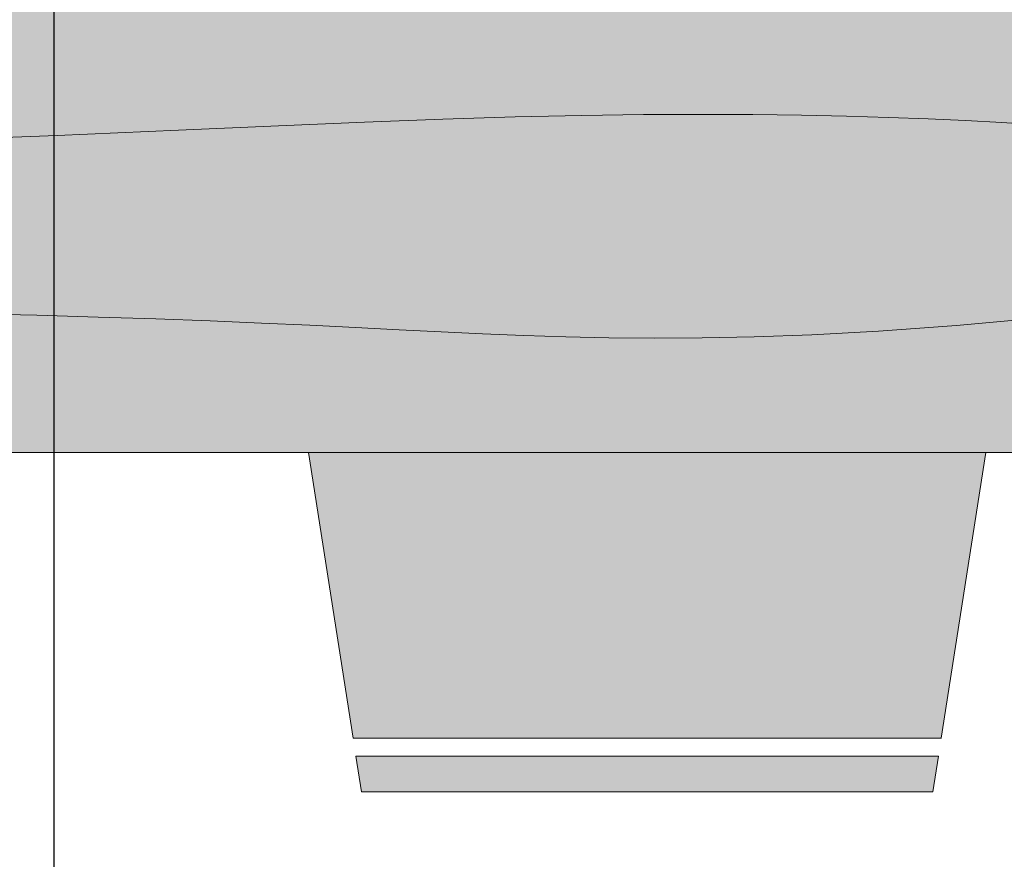
# Model space of a CAD drawing. Units: inches. Extents: x 2549 to 3108, y 1683 to 2362.
# Tile 11 of 30: x 2734.13 to 2749, y 2015.6 to 2028.28. Entities that reach past the tile are written whole.
import ezdxf

# ---------------------------------------------------------------- set-up
doc = ezdxf.new("R2010")
doc.units = ezdxf.units.IN
for name, color, linetype, lineweight in [('A-ANNO-DIMS', 2, 'Continuous', 18), ('A-FURN', 8, 'Continuous', 18), ('A-FURN-PATT', 9, 'Continuous', 13)]:
    doc.layers.add(name, color=color, linetype=linetype, lineweight=lineweight)
doc.layers.add('C-PKNG-VEHI-PATT', color=251, linetype='Continuous', lineweight=13, true_color=0x636466)
doc.layers.add('C-PVMT-PATT', color=9, linetype='Continuous', lineweight=13, true_color=0xc7c8ca)
doc.styles.get("Standard").update_dxf_attribs({"font": 'arial.ttf'})
doc.dimstyles.get("Standard").update_dxf_attribs({"dimtxt": 0.18, "dimasz": 0.18, "dimexe": 0.18, "dimexo": 0.0625, "dimgap": 0.09, "dimtad": 0, "dimtih": 1, "dimtoh": 1, "dimdec": 4, "dimzin": 0, "dimdsep": 46, "dimtxsty": 'Standard', "dimcen": 0.09, "dimadec": 0, "dimazin": 0, "dimtfac": 1, "dimtdec": 4, "dimtofl": 0, "dimtmove": 0, "dimatfit": 3, "dimfxl": 1, "dimtolj": 1, "dimtzin": 0, "dimarcsym": 0})

# ---------------------------------------------------------------- blocks, each defined once
blk = doc.blocks.new('Dining Set - 36 x 72 in.')
for p, q in [((-36, -18), (36, -18)), ((5.7657, -26.0006), (4.5153, -17.99762)), ((23.4848, -17.99762), (22.2345, -25.99928)), ((5.7696, -26), (22.2392, -26)), ((6, -27.5), (5.8438, -26.50044)), ((22.1584, -26.5), (5.8466, -26.5)), ((22.1563, -26.49967), (22, -27.5)), ((6, -27.5), (22, -27.5))]:
    blk.add_line(p, q)
for points in [[(-6.7396, -9.28125), (-2.5226, -9.12354), (0.8789, -8.98047), (3.6769, -8.85498), (6.0833, -8.75), (8.2767, -8.66765), (10.3021, -8.60677), (12.1712, -8.56543), (13.8958, -8.54167), (15.4876, -8.53353), (16.9583, -8.53907), (18.3197, -8.55632), (19.5834, -8.58334), (20.7616, -8.61841), (21.8685, -8.66081), (22.9188, -8.71004), (23.9271, -8.76563), (24.9081, -8.82707)], [(-4.9224, -14.11833), (-3.0905, -14.16016), (-1.3709, -14.20785), (0.2448, -14.26042), (1.7647, -14.3169), (3.1973, -14.3763), (4.5507, -14.43767), (5.8333, -14.5), (7.0554, -14.5621), (8.235, -14.62175), (9.3922, -14.67652), (10.5469, -14.72396), (11.7192, -14.76164), (12.929, -14.78711), (14.1965, -14.79794), (15.5417, -14.79167), (16.9933, -14.76424), (18.6152, -14.70508), (20.4804, -14.60197), (22.6615, -14.44271), (25.2312, -14.21509), (28.2624, -13.9069), (31.8277, -13.50594), (36, -13)]]:
    blk.add_lwpolyline(points)
blk = doc.blocks.new('*D43')
at = {"layer": 'A-ANNO-DIMS', "color": 0, "lineweight": -2, "transparency": 16777216}
for p, q in [((2734.643, 2080.461), (2734.643, 1683.444)), ((2806.643, 2080.461), (2806.643, 1683.444)), ((2734.823, 1683.624), (2770.425, 1683.624)), ((2806.463, 1683.624), (2770.86, 1683.624))]:
    blk.add_line(p, q, dxfattribs=at)
at = {"layer": 'A-ANNO-DIMS', "color": 0, "transparency": 16777216}
for points in [[(2734.823, 1683.654), (2734.823, 1683.594), (2734.643, 1683.624)], [(2806.463, 1683.654), (2806.463, 1683.594), (2806.643, 1683.624)]]:
    blk.add_solid(points, dxfattribs=at)
at = {"layer": 'Defpoints', "color": 0, "transparency": 16777216}
for p in [(2734.643, 2080.524), (2806.643, 2080.524), (2806.643, 1683.624)]:
    blk.add_point(p, dxfattribs=at)
at = {"layer": 'A-ANNO-DIMS', "color": 0, "transparency": 16777216, "insert": (2770.643, 1683.624), "char_height": 0.18, "attachment_point": 5}
blk.add_mtext('\\A1;72', dxfattribs=at)
blk = doc.blocks.new('*D44')
at = {"layer": 'A-ANNO-DIMS', "color": 0, "lineweight": -2, "transparency": 16777216}
for p, q in [((2662.643, 2040.993), (2662.643, 1683.444)), ((2806.643, 2016.129), (2806.643, 1683.444)), ((2662.823, 1683.624), (2734.363, 1683.624)), ((2806.463, 1683.624), (2734.923, 1683.624))]:
    blk.add_line(p, q, dxfattribs=at)
at = {"layer": 'A-ANNO-DIMS', "color": 0, "transparency": 16777216}
for points in [[(2662.823, 1683.654), (2662.823, 1683.594), (2662.643, 1683.624)], [(2806.463, 1683.654), (2806.463, 1683.594), (2806.643, 1683.624)]]:
    blk.add_solid(points, dxfattribs=at)
at = {"layer": 'Defpoints', "color": 0, "transparency": 16777216}
for p in [(2662.643, 2041.056), (2806.643, 2016.191), (2806.643, 1683.624)]:
    blk.add_point(p, dxfattribs=at)
at = {"layer": 'A-ANNO-DIMS', "color": 0, "transparency": 16777216, "insert": (2734.643, 1683.624), "char_height": 0.18, "attachment_point": 5}
blk.add_mtext('\\A1;144', dxfattribs=at)
blk = doc.blocks.new('*D59')
at = {"layer": 'A-ANNO-DIMS', "color": 0, "lineweight": -2, "transparency": 16777216}
for p, q in [((2680.978, 1761.586), (2680.978, 2362.323)), ((2786.158, 1761.586), (2786.158, 2362.323)), ((2681.158, 2362.143), (2733.112, 2362.143)), ((2785.978, 2362.143), (2734.023, 2362.143))]:
    blk.add_line(p, q, dxfattribs=at)
at = {"layer": 'A-ANNO-DIMS', "color": 0, "transparency": 16777216}
for points in [[(2681.158, 2362.173), (2681.158, 2362.113), (2680.978, 2362.143)], [(2785.978, 2362.173), (2785.978, 2362.113), (2786.158, 2362.143)]]:
    blk.add_solid(points, dxfattribs=at)
at = {"layer": 'Defpoints', "color": 0, "transparency": 16777216}
for p in [(2786.158, 2362.143), (2680.978, 1761.524), (2786.158, 1761.524)]:
    blk.add_point(p, dxfattribs=at)
at = {"layer": 'A-ANNO-DIMS', "color": 0, "transparency": 16777216, "insert": (2733.568, 2362.143), "char_height": 0.18, "attachment_point": 5}
blk.add_mtext('\\A1;105.18', dxfattribs=at)

msp = doc.modelspace()

# ---------------------------------------------------------------- hatches: boundary and pattern name
at = {"layer": 'A-FURN-PATT'}
h = msp.add_hatch(color=256, dxfattribs=at)
h.dxf.hatch_style = 1
h.paths.add_polyline_path([(2732.9458, 2045.4744), (2724.0631, 2045.4744), (2723.389, 2041.1594), (2733.6201, 2041.1594)])
h.paths.add_polyline_path([(2748.0481, 2045.4744), (2739.1654, 2045.4744), (2738.4912, 2041.1594), (2748.7223, 2041.1594)])
h.paths.add_polyline_path([(2747.9217, 2046.2834), (2739.2918, 2046.2834), (2739.2075, 2045.7441), (2748.006, 2045.7441)])
h.paths.add_polyline_path([(2732.8194, 2046.2834), (2724.1896, 2046.2834), (2724.1053, 2045.7441), (2732.9037, 2045.7441)])
h.paths.add_polyline_path([(2759.7877, 2035.8922), (2755.4728, 2036.5664), (2755.4728, 2026.3353), (2759.7877, 2027.0095)])
h.paths.add_polyline_path([(2760.5968, 2035.7658), (2760.0574, 2035.8501), (2760.0574, 2027.0516), (2760.5968, 2027.1359)])
h.paths.add_polyline_path([(2716.6384, 2036.5664), (2712.3235, 2035.8922), (2712.3235, 2027.0095), (2716.6384, 2026.3353)])
h.paths.add_polyline_path([(2733.6201, 2021.7423), (2723.389, 2021.7423), (2724.0631, 2017.4273), (2732.9458, 2017.4273)])
h.paths.add_polyline_path([(2748.7223, 2021.7423), (2738.4912, 2021.7423), (2739.1654, 2017.4273), (2748.0481, 2017.4273)])
h.paths.add_polyline_path([(2748.006, 2017.1576), (2739.2075, 2017.1576), (2739.2918, 2016.6183), (2747.9217, 2016.6183)])
h.paths.add_polyline_path([(2732.9037, 2017.1576), (2724.1053, 2017.1576), (2724.1896, 2016.6183), (2732.8194, 2016.6183)])
h.paths.add_polyline_path([(2712.0538, 2035.85), (2711.5145, 2035.7658), (2711.5145, 2027.1359), (2712.0538, 2027.0516)])
h = msp.add_hatch(color=256, dxfattribs=at)
h.dxf.hatch_style = 1
h.paths.add_polyline_path([(2744.8667, 2037.254), (2744.7754, 2037.3839), (2744.7125, 2037.4849), (2744.6595, 2037.5854), (2744.5963, 2037.7375), (2744.5695, 2037.9287), (2744.6003, 2038.0617), (2744.6406, 2038.148), (2744.7014, 2038.2298), (2744.7817, 2038.3053), (2744.8799, 2038.3724), (2744.9945, 2038.4289), (2745.1238, 2038.4728), (2745.2663, 2038.5019), (2745.4204, 2038.5142), (2745.5844, 2038.5076), (2745.7585, 2038.4805), (2745.9486, 2038.4342), (2746.1624, 2038.3705), (2746.4075, 2038.2913), (2746.6917, 2038.1983), (2747.0224, 2038.0936), (2747.4074, 2037.9788), (2747.8543, 2037.8558), (2748.3724, 2037.7256), (2748.9783, 2037.5851), (2749.69, 2037.4304), (2750.5258, 2037.2575), (2751.5038, 2037.0624), (2752.6422, 2036.8414), (2753.9591, 2036.5902), (2755.4728, 2036.3051), (2755.4728, 2039.002), (2754.0892, 2039.103), (2752.7721, 2039.2035), (2751.5251, 2039.303), (2750.3516, 2039.4009), (2749.255, 2039.4967), (2748.2388, 2039.5898), (2747.3063, 2039.6798), (2746.4609, 2039.7661), (2745.7045, 2039.8482), (2745.0321, 2039.9255), (2744.4371, 2039.9976), (2743.9129, 2040.0639), (2743.4531, 2040.1238), (2743.0509, 2040.1769), (2742.6998, 2040.2227), (2742.3932, 2040.2605), (2742.1251, 2040.29), (2741.8917, 2040.3111), (2741.69, 2040.3237), (2741.5167, 2040.3279), (2741.3687, 2040.3237), (2741.2428, 2040.3111), (2741.1359, 2040.29), (2741.0448, 2040.2605), (2740.9668, 2040.2227), (2740.9015, 2040.1776), (2740.8488, 2040.1262), (2740.8088, 2040.0695), (2740.7814, 2040.0085), (2740.7667, 2039.9445), (2740.7646, 2039.8783), (2740.7751, 2039.811), (2740.7978, 2039.7435), (2740.8306, 2039.6755), (2740.8707, 2039.6064), (2740.9155, 2039.5357), (2740.996, 2039.4111), (2741.0771, 2039.2637), (2741.1346, 2039.0945), (2741.1499, 2038.9139), (2741.1092, 2038.7391), (2741.0289, 2038.6239), (2740.9549, 2038.5525), (2740.8586, 2038.4895), (2740.733, 2038.4359), (2740.5693, 2038.3929), (2740.3593, 2038.3615), (2740.0946, 2038.3427), (2739.7666, 2038.3376), (2739.367, 2038.3473), (2738.8873, 2038.3727), (2738.3203, 2038.4145), (2737.6635, 2038.471), (2736.9156, 2038.5402), (2736.0753, 2038.6199), (2735.1412, 2038.7081), (2734.112, 2038.8025), (2732.9864, 2038.9012), (2731.7632, 2039.002), (2730.4376, 2039.1026), (2728.9922, 2039.2), (2727.4062, 2039.2911), (2725.6588, 2039.3728), (2723.7291, 2039.4418), (2721.5964, 2039.495), (2719.2397, 2039.5292), (2716.6384, 2039.5413), (2716.6384, 2036.8445), (2720.4266, 2036.9215), (2723.5572, 2036.9548), (2726.1183, 2036.9512), (2728.1983, 2036.9175), (2729.8853, 2036.8608), (2731.2677, 2036.7876), (2732.4336, 2036.705), (2733.4711, 2036.6198), (2734.4538, 2036.5375), (2735.3951, 2036.4589), (2736.2938, 2036.3835), (2737.1484, 2036.3108), (2737.9578, 2036.2401), (2738.7205, 2036.171), (2739.4353, 2036.103), (2740.1009, 2036.0355), (2740.7163, 2035.9683), (2741.2828, 2035.9027), (2741.8019, 2035.8403), (2742.2752, 2035.7826), (2742.7042, 2035.7313), (2743.0906, 2035.6878), (2743.4358, 2035.6539), (2743.7416, 2035.6309), (2744.0097, 2035.6203), (2744.243, 2035.6218), (2744.4448, 2035.6349), (2744.6181, 2035.659), (2744.7661, 2035.6937), (2744.892, 2035.7384), (2744.9989, 2035.7926), (2745.09, 2035.8557), (2745.1679, 2035.9271), (2745.2326, 2036.006), (2745.2836, 2036.0911), (2745.3204, 2036.1815), (2745.3424, 2036.2762), (2745.3492, 2036.374), (2745.3401, 2036.4739), (2745.3148, 2036.5748), (2745.2731, 2036.676), (2745.2178, 2036.7771), (2745.152, 2036.8782), (2745.0788, 2036.9794), (2745.0013, 2037.0805)])
h.paths.add_polyline_path([(2755.4728, 2036.3051), (2753.9591, 2036.5902), (2752.6422, 2036.8414), (2751.5038, 2037.0624), (2750.5258, 2037.2575), (2749.69, 2037.4304), (2748.9783, 2037.5851), (2748.3724, 2037.7256), (2747.8543, 2037.8558), (2747.4074, 2037.9788), (2747.0224, 2038.0936), (2746.6917, 2038.1983), (2746.4075, 2038.2913), (2746.1624, 2038.3705), (2745.9486, 2038.4342), (2745.7585, 2038.4805), (2745.5844, 2038.5076), (2745.4204, 2038.5142), (2745.2663, 2038.5019), (2745.1238, 2038.4728), (2744.9945, 2038.4289), (2744.8799, 2038.3724), (2744.7817, 2038.3053), (2744.7014, 2038.2298), (2744.6406, 2038.148), (2744.6003, 2038.0617), (2744.5794, 2037.9717), (2744.5765, 2037.8786), (2744.59, 2037.7828), (2744.6182, 2037.6849), (2744.6595, 2037.5854), (2744.7125, 2037.4849), (2744.7754, 2037.3839), (2744.8465, 2037.2827), (2744.9229, 2037.1816), (2745.0013, 2037.0805), (2745.1278, 2036.9154), (2745.2178, 2036.7771), (2745.2731, 2036.676), (2745.3148, 2036.5748), (2745.3401, 2036.4739), (2745.3492, 2036.374), (2745.3424, 2036.2762), (2745.3204, 2036.1815), (2745.2836, 2036.0911), (2745.2326, 2036.006), (2745.1679, 2035.9271), (2745.09, 2035.8557), (2744.9989, 2035.7926), (2744.892, 2035.7384), (2744.7661, 2035.6937), (2744.6181, 2035.659), (2744.4448, 2035.6349), (2744.243, 2035.6218), (2744.0097, 2035.6203), (2743.7416, 2035.6309), (2743.4358, 2035.6539), (2743.0906, 2035.6878), (2742.7042, 2035.7313), (2742.2752, 2035.7826), (2741.8019, 2035.8403), (2741.2828, 2035.9027), (2740.7163, 2035.9683), (2740.1009, 2036.0355), (2739.4353, 2036.103), (2738.7205, 2036.171), (2737.9578, 2036.2401), (2737.1484, 2036.3108), (2736.2938, 2036.3835), (2735.3951, 2036.4589), (2734.4538, 2036.5375), (2733.4711, 2036.6198), (2732.4336, 2036.705), (2731.2677, 2036.7876), (2729.8853, 2036.8608), (2728.1983, 2036.9175), (2726.1183, 2036.9512), (2723.5572, 2036.9548), (2720.4266, 2036.9215), (2716.6384, 2036.8445), (2716.6384, 2034.4174), (2719.4886, 2034.3283), (2721.9949, 2034.2608), (2724.1925, 2034.2112), (2726.1167, 2034.1758), (2727.8028, 2034.1509), (2729.2861, 2034.1329), (2730.602, 2034.1181), (2731.7856, 2034.1027), (2732.8685, 2034.0839), (2733.8666, 2034.0613), (2734.7919, 2034.0356), (2735.6567, 2034.0072), (2736.473, 2033.9768), (2737.253, 2033.9447), (2738.0088, 2033.9116), (2738.7525, 2033.878), (2739.493, 2033.8445), (2740.2273, 2033.812), (2740.9489, 2033.7816), (2741.6515, 2033.7544), (2742.3289, 2033.7314), (2742.9747, 2033.7137), (2743.5825, 2033.7022), (2744.1461, 2033.6982), (2744.6607, 2033.7024), (2745.1272, 2033.7151), (2745.5485, 2033.7361), (2745.9272, 2033.7656), (2746.2658, 2033.8036), (2746.567, 2033.8499), (2746.8334, 2033.9047), (2747.0677, 2033.9679), (2747.2728, 2034.0393), (2747.4525, 2034.1175), (2747.6113, 2034.201), (2747.7531, 2034.2881), (2747.8824, 2034.3774), (2748.0032, 2034.4672), (2748.1197, 2034.556), (2748.2363, 2034.6421), (2748.3567, 2034.7241), (2748.4828, 2034.8008), (2748.6163, 2034.8712), (2748.7588, 2034.9343), (2748.9118, 2034.9889), (2749.077, 2035.034), (2749.2558, 2035.0686), (2749.4499, 2035.0916), (2749.6603, 2035.1022), (2749.8861, 2035.1007), (2750.1254, 2035.0876), (2750.3769, 2035.0635), (2750.639, 2035.0288), (2750.91, 2034.9841), (2751.1884, 2034.93), (2751.4725, 2034.8668), (2751.7642, 2034.7949), (2752.0786, 2034.7123), (2752.4341, 2034.6172), (2752.849, 2034.5073), (2753.3419, 2034.3805), (2753.9313, 2034.2348), (2754.6354, 2034.068), (2755.4728, 2033.878)])
h.paths.add_polyline_path([(2755.4728, 2033.878), (2754.6354, 2034.068), (2753.9313, 2034.2348), (2753.3419, 2034.3805), (2752.849, 2034.5073), (2752.4341, 2034.6172), (2752.0786, 2034.7123), (2751.7642, 2034.7949), (2751.4725, 2034.8668), (2751.1884, 2034.93), (2750.91, 2034.9841), (2750.639, 2035.0288), (2750.3769, 2035.0635), (2750.1254, 2035.0876), (2749.8861, 2035.1007), (2749.6603, 2035.1022), (2749.4499, 2035.0916), (2749.2558, 2035.0686), (2749.077, 2035.034), (2748.9118, 2034.9889), (2748.7588, 2034.9343), (2748.6163, 2034.8712), (2748.4828, 2034.8008), (2748.3567, 2034.7241), (2748.2363, 2034.6421), (2748.1197, 2034.556), (2748.0032, 2034.4672), (2747.8824, 2034.3774), (2747.7531, 2034.2881), (2747.6113, 2034.201), (2747.4525, 2034.1175), (2747.2728, 2034.0393), (2747.0677, 2033.9679), (2746.8334, 2033.9047), (2746.567, 2033.8499), (2746.2658, 2033.8036), (2745.9272, 2033.7656), (2745.5485, 2033.7361), (2745.1272, 2033.7151), (2744.6607, 2033.7024), (2744.1461, 2033.6982), (2743.5825, 2033.7022), (2742.9747, 2033.7137), (2742.3289, 2033.7314), (2741.6515, 2033.7544), (2740.9489, 2033.7816), (2740.2273, 2033.812), (2739.493, 2033.8445), (2738.7525, 2033.878), (2738.0088, 2033.9116), (2737.253, 2033.9447), (2736.473, 2033.9768), (2735.6567, 2034.0072), (2734.7919, 2034.0356), (2733.8666, 2034.0613), (2732.8685, 2034.0839), (2731.7856, 2034.1027), (2730.602, 2034.1181), (2729.2861, 2034.1329), (2727.8028, 2034.1509), (2726.1167, 2034.1758), (2724.1925, 2034.2112), (2721.9949, 2034.2608), (2719.4886, 2034.3283), (2716.6384, 2034.4174), (2716.6384, 2030.9115), (2719.4477, 2031.0954), (2722.0216, 2031.2447), (2724.3773, 2031.363), (2726.5324, 2031.4537), (2728.5042, 2031.5201), (2730.3101, 2031.5657), (2731.9674, 2031.5939), (2733.4936, 2031.6082), (2734.9046, 2031.6115), (2736.2109, 2031.6057), (2737.4211, 2031.592), (2738.5446, 2031.5716), (2739.59, 2031.5461), (2740.5665, 2031.5165), (2741.4829, 2031.4843), (2742.3482, 2031.4509), (2743.1698, 2031.4174), (2743.9488, 2031.3855), (2744.6845, 2031.3568), (2745.3766, 2031.3329), (2746.0244, 2031.3152), (2746.6274, 2031.3055), (2747.1851, 2031.3052), (2747.697, 2031.316), (2748.1634, 2031.3388), (2748.5882, 2031.3722), (2748.9761, 2031.414), (2749.3319, 2031.4621), (2749.6603, 2031.5144), (2749.9661, 2031.5688), (2750.254, 2031.6233), (2750.5287, 2031.6756), (2750.7946, 2031.7239), (2751.0553, 2031.7669), (2751.314, 2031.8036), (2751.5737, 2031.8329), (2751.8375, 2031.8538), (2752.1088, 2031.8652), (2752.3906, 2031.8661), (2752.6861, 2031.8554), (2752.9965, 2031.8326), (2753.315, 2031.7999), (2753.633, 2031.7598), (2753.9418, 2031.7149), (2754.2327, 2031.6679), (2754.497, 2031.6215), (2754.7259, 2031.5782), (2754.911, 2031.5407), (2755.0467, 2031.5111), (2755.141, 2031.4888), (2755.2053, 2031.4728), (2755.2509, 2031.4621), (2755.2891, 2031.4556), (2755.3313, 2031.4523), (2755.3888, 2031.451), (2755.4728, 2031.4509)])
h.paths.add_polyline_path([(2743.9488, 2031.3855), (2743.1698, 2031.4174), (2742.3482, 2031.4509), (2741.4829, 2031.4843), (2740.5665, 2031.5165), (2739.59, 2031.5461), (2738.5446, 2031.5716), (2737.4211, 2031.592), (2736.2109, 2031.6057), (2734.9046, 2031.6115), (2733.4936, 2031.6082), (2731.9674, 2031.5939), (2730.3101, 2031.5657), (2728.5042, 2031.5201), (2726.5324, 2031.4537), (2724.3773, 2031.363), (2722.0216, 2031.2447), (2719.4477, 2031.0954), (2716.6384, 2030.9115), (2716.6384, 2027.945), (2721.3933, 2028.046), (2725.223, 2028.1465), (2728.2515, 2028.246), (2730.603, 2028.3439), (2732.4013, 2028.4397), (2733.7707, 2028.5328), (2734.8351, 2028.6228), (2735.7185, 2028.7091), (2736.5253, 2028.7912), (2737.2808, 2028.8692), (2737.9904, 2028.9429), (2738.6597, 2029.0125), (2739.2943, 2029.0778), (2739.8997, 2029.1389), (2740.4813, 2029.1958), (2741.0448, 2029.2484), (2741.5952, 2029.2967), (2742.1361, 2029.3397), (2742.6708, 2029.3764), (2743.2022, 2029.4058), (2743.7337, 2029.4266), (2744.2683, 2029.4381), (2744.8093, 2029.4389), (2745.3597, 2029.4282), (2745.9213, 2029.4053), (2746.4897, 2029.3713), (2747.0592, 2029.3279), (2747.6239, 2029.2765), (2748.1781, 2029.2189), (2748.716, 2029.1564), (2749.2317, 2029.0909), (2749.7196, 2029.0237), (2750.1754, 2028.9563), (2750.602, 2028.8892), (2751.0039, 2028.8226), (2751.3854, 2028.7568), (2751.7512, 2028.6921), (2752.1057, 2028.6287), (2752.4532, 2028.5668), (2752.7985, 2028.5068), (2753.1447, 2028.4496), (2753.4913, 2028.399), (2753.8363, 2028.3595), (2754.1778, 2028.3355), (2754.514, 2028.3315), (2754.8432, 2028.352), (2755.1634, 2028.4014), (2755.4728, 2028.4843), (2755.4728, 2031.4509), (2755.3151, 2031.4512), (2755.2429, 2031.4634), (2755.141, 2031.4888), (2755.0467, 2031.5111), (2754.911, 2031.5407), (2754.7259, 2031.5782), (2754.497, 2031.6215), (2754.2327, 2031.6679), (2753.9418, 2031.7149), (2753.633, 2031.7598), (2753.315, 2031.7999), (2752.9965, 2031.8326), (2752.6861, 2031.8554), (2752.3906, 2031.8661), (2752.1088, 2031.8652), (2751.8375, 2031.8538), (2751.5737, 2031.8329), (2751.314, 2031.8036), (2751.0553, 2031.7669), (2750.7946, 2031.7239), (2750.5287, 2031.6756), (2750.254, 2031.6233), (2749.9661, 2031.5688), (2749.6603, 2031.5144), (2749.3319, 2031.4621), (2748.9761, 2031.414), (2748.5882, 2031.3722), (2748.1634, 2031.3388), (2747.697, 2031.316), (2747.1851, 2031.3052), (2746.6274, 2031.3055), (2746.0244, 2031.3152), (2745.3766, 2031.3329), (2744.6845, 2031.3568)])
h.paths.add_polyline_path([(2755.4728, 2028.4843), (2755.1634, 2028.4014), (2754.8432, 2028.352), (2754.514, 2028.3315), (2754.1778, 2028.3355), (2753.8363, 2028.3595), (2753.4913, 2028.399), (2753.1447, 2028.4496), (2752.7985, 2028.5068), (2752.4532, 2028.5668), (2752.1057, 2028.6287), (2751.7512, 2028.6921), (2751.3854, 2028.7568), (2751.0039, 2028.8226), (2750.602, 2028.8892), (2750.1754, 2028.9563), (2749.7196, 2029.0237), (2749.2317, 2029.0909), (2748.716, 2029.1564), (2748.1781, 2029.2189), (2747.6239, 2029.2765), (2747.0592, 2029.3279), (2746.4897, 2029.3713), (2745.9213, 2029.4053), (2745.3597, 2029.4282), (2744.8093, 2029.4389), (2744.2683, 2029.4381), (2743.7337, 2029.4266), (2743.2022, 2029.4058), (2742.6708, 2029.3764), (2742.1361, 2029.3397), (2741.5952, 2029.2967), (2741.0448, 2029.2484), (2740.4813, 2029.1958), (2739.8997, 2029.1389), (2739.2943, 2029.0778), (2738.6597, 2029.0125), (2737.9904, 2028.9429), (2737.2808, 2028.8692), (2736.5253, 2028.7912), (2735.7185, 2028.7091), (2734.8351, 2028.6228), (2733.7707, 2028.5328), (2732.4013, 2028.4397), (2730.603, 2028.3439), (2728.2515, 2028.246), (2725.223, 2028.1465), (2721.3933, 2028.046), (2716.6384, 2027.945), (2716.6384, 2023.63), (2719.8271, 2023.719), (2722.5536, 2023.7853), (2724.8739, 2023.8315), (2726.8443, 2023.8604), (2728.5207, 2023.8745), (2729.9593, 2023.8765), (2731.2162, 2023.8691), (2732.3475, 2023.8548), (2733.4006, 2023.8359), (2734.3887, 2023.8133), (2735.3162, 2023.7876), (2736.1877, 2023.7593), (2737.0074, 2023.7288), (2737.7801, 2023.6968), (2738.5101, 2023.6637), (2739.2019, 2023.63), (2739.8611, 2023.5965), (2740.4973, 2023.5644), (2741.1215, 2023.5348), (2741.7443, 2023.5092), (2742.3766, 2023.4889), (2743.0291, 2023.4752), (2743.7127, 2023.4693), (2744.4383, 2023.4727), (2745.2212, 2023.4875), (2746.096, 2023.5194), (2747.1021, 2023.575), (2748.2785, 2023.6609), (2749.6645, 2023.7837), (2751.2994, 2023.9499), (2753.2224, 2024.1662), (2755.4728, 2024.4391)])
h.paths.add_polyline_path([(2755.4728, 2026.3269), (2754.9554, 2026.3329), (2754.418, 2026.3497), (2753.8658, 2026.3755), (2753.3041, 2026.4083), (2752.7382, 2026.4465), (2752.1734, 2026.4881), (2751.6149, 2026.5312), (2751.068, 2026.5741), (2750.5357, 2026.6151), (2750.0124, 2026.6538), (2749.4902, 2026.6898), (2748.9611, 2026.723), (2748.4173, 2026.753), (2747.8508, 2026.7795), (2747.2537, 2026.8024), (2746.6182, 2026.8213), (2745.9367, 2026.8359), (2745.2024, 2026.8452), (2744.4091, 2026.8482), (2743.5505, 2026.8438), (2742.6204, 2026.8309), (2741.6122, 2026.8087), (2740.5198, 2026.7758), (2739.3368, 2026.7314), (2738.0388, 2026.6748), (2736.5297, 2026.6071), (2734.695, 2026.5299), (2732.4205, 2026.4449), (2729.5919, 2026.3535), (2726.0949, 2026.2573), (2721.8152, 2026.1581), (2716.6384, 2026.0572), (2716.6384, 2023.63), (2719.8271, 2023.719), (2722.5536, 2023.7853), (2724.8739, 2023.8315), (2726.8443, 2023.8604), (2728.5207, 2023.8745), (2729.9593, 2023.8765), (2731.2162, 2023.8691), (2732.3475, 2023.8548), (2733.4006, 2023.8359), (2734.3887, 2023.8133), (2735.3162, 2023.7876), (2736.1877, 2023.7593), (2737.0074, 2023.7288), (2737.7801, 2023.6968), (2738.5101, 2023.6637), (2739.2019, 2023.63), (2739.8611, 2023.5965), (2740.4973, 2023.5644), (2741.1215, 2023.5348), (2741.7443, 2023.5092), (2742.3766, 2023.4889), (2743.0291, 2023.4752), (2743.7127, 2023.4693), (2744.4383, 2023.4727), (2745.2212, 2023.4875), (2746.096, 2023.5194), (2747.1021, 2023.575), (2748.2785, 2023.6609), (2749.6645, 2023.7837), (2751.2994, 2023.9499), (2753.2224, 2024.1662), (2755.4728, 2024.4391)], flags=17)
h.paths.add_polyline_path([(2740.4973, 2023.5644), (2739.8611, 2023.5965), (2739.2019, 2023.63), (2738.5101, 2023.6637), (2737.7801, 2023.6968), (2737.0074, 2023.7288), (2736.1877, 2023.7593), (2735.3162, 2023.7876), (2734.3887, 2023.8133), (2733.4006, 2023.8359), (2732.3475, 2023.8548), (2731.2162, 2023.8691), (2729.9593, 2023.8765), (2728.5207, 2023.8745), (2726.8443, 2023.8604), (2724.8739, 2023.8315), (2722.5536, 2023.7853), (2719.8271, 2023.719), (2716.6384, 2023.63), (2716.6384, 2021.7423), (2755.4728, 2021.7423), (2755.4728, 2024.4391), (2753.2224, 2024.1662), (2751.2994, 2023.9499), (2749.6645, 2023.7837), (2748.2785, 2023.6609), (2747.1021, 2023.575), (2746.096, 2023.5194), (2745.2212, 2023.4875), (2744.4383, 2023.4727), (2743.7127, 2023.4693), (2743.0291, 2023.4752), (2742.3766, 2023.4889), (2741.7443, 2023.5092), (2741.1215, 2023.5348)])
h.paths.add_polyline_path([(2741.1359, 2040.29), (2741.2428, 2040.3111), (2741.3687, 2040.3237), (2741.5167, 2040.3279), (2741.69, 2040.3237), (2741.8917, 2040.3111), (2742.1251, 2040.29), (2742.3932, 2040.2605), (2742.6998, 2040.2227), (2743.0509, 2040.1769), (2743.4531, 2040.1238), (2743.9129, 2040.0639), (2744.4371, 2039.9976), (2745.0321, 2039.9255), (2745.7045, 2039.8482), (2746.4609, 2039.7661), (2747.3063, 2039.6798), (2748.2388, 2039.5898), (2749.255, 2039.4967), (2750.3516, 2039.4009), (2751.5251, 2039.303), (2752.7721, 2039.2035), (2754.0892, 2039.103), (2755.4728, 2039.002), (2755.4728, 2041.1594), (2716.6384, 2041.1594), (2716.6384, 2039.5413), (2719.2397, 2039.5292), (2721.5964, 2039.495), (2723.7291, 2039.4418), (2725.6588, 2039.3728), (2727.4062, 2039.2911), (2728.9922, 2039.2), (2730.4376, 2039.1026), (2731.7632, 2039.002), (2732.9864, 2038.9012), (2734.112, 2038.8025), (2735.1412, 2038.7081), (2736.0753, 2038.6199), (2736.9156, 2038.5402), (2737.6635, 2038.471), (2738.3203, 2038.4145), (2738.8873, 2038.3727), (2739.367, 2038.3473), (2739.7666, 2038.3376), (2740.0946, 2038.3427), (2740.3593, 2038.3615), (2740.5693, 2038.3929), (2740.733, 2038.4359), (2740.8586, 2038.4895), (2740.9549, 2038.5525), (2741.0289, 2038.6239), (2741.0834, 2038.7021), (2741.12, 2038.7856), (2741.1403, 2038.8728), (2741.1458, 2038.962), (2741.1382, 2039.0518), (2741.1189, 2039.1406), (2741.0897, 2039.2267), (2741.0522, 2039.309), (2741.0089, 2039.3875), (2740.9625, 2039.4629), (2740.8772, 2039.5951), (2740.8072, 2039.7159), (2740.7635, 2039.8453), (2740.7677, 2039.9782), (2740.8229, 2040.1009), (2740.9289, 2040.2044), (2741.0448, 2040.2605)])
h = msp.add_hatch(color=256, dxfattribs=at)
h.dxf.hatch_style = 1
h.paths.add_polyline_path([(2755.4728, 2026.3269), (2754.9554, 2026.3329), (2754.418, 2026.3497), (2753.8658, 2026.3755), (2753.3041, 2026.4083), (2752.7382, 2026.4465), (2752.1734, 2026.4881), (2751.6149, 2026.5312), (2751.068, 2026.5741), (2750.5357, 2026.6151), (2750.0124, 2026.6538), (2749.4902, 2026.6898), (2748.9611, 2026.723), (2748.4173, 2026.753), (2747.8508, 2026.7795), (2747.2537, 2026.8024), (2746.6182, 2026.8213), (2745.9367, 2026.8359), (2745.2024, 2026.8452), (2744.4091, 2026.8482), (2743.5505, 2026.8438), (2742.6204, 2026.8309), (2741.6122, 2026.8087), (2740.5198, 2026.7758), (2739.3368, 2026.7314), (2738.0388, 2026.6748), (2736.5297, 2026.6071), (2734.695, 2026.5299), (2732.4205, 2026.4449), (2729.5919, 2026.3535), (2726.0949, 2026.2573), (2721.8152, 2026.1581), (2716.6384, 2026.0572), (2716.6384, 2023.63), (2719.8271, 2023.719), (2722.5536, 2023.7853), (2724.8739, 2023.8315), (2726.8443, 2023.8604), (2728.5207, 2023.8745), (2729.9593, 2023.8765), (2731.2162, 2023.8691), (2732.3475, 2023.8548), (2733.4006, 2023.8359), (2734.3887, 2023.8133), (2735.3162, 2023.7876), (2736.1877, 2023.7593), (2737.0074, 2023.7288), (2737.7801, 2023.6968), (2738.5101, 2023.6637), (2739.2019, 2023.63), (2739.8611, 2023.5965), (2740.4973, 2023.5644), (2741.1215, 2023.5348), (2741.7443, 2023.5092), (2742.3766, 2023.4889), (2743.0291, 2023.4752), (2743.7127, 2023.4693), (2744.4383, 2023.4727), (2745.2212, 2023.4875), (2746.096, 2023.5194), (2747.1021, 2023.575), (2748.2785, 2023.6609), (2749.6645, 2023.7837), (2751.2994, 2023.9499), (2753.2224, 2024.1662), (2755.4728, 2024.4391)])
at = {"layer": 'C-PKNG-VEHI-PATT'}
h = msp.add_hatch(color=256, dxfattribs=at)
h.dxf.hatch_style = 1
edge = h.paths.add_edge_path()
edge.add_ellipse((2935.7258, 1791.964), major_axis=(-50.66, 0), ratio=0.8423039, start_angle=248.16505, end_angle=265.72258)
edge.add_line((2938.911, 1834.5507), (2925.8653, 1834.5507))
edge.add_ellipse((2929.0505, 1791.964), major_axis=(50.66, 0), ratio=0.8423039, start_angle=94.27742, end_angle=111.83495)
edge.add_line((2912.8508, 1832.3947), (2914.2044, 1822.2495))
edge.add_ellipse((2930.6538, 1783.1023), major_axis=(-49.3014, 0), ratio=0.8423039, start_angle=-85.12993, end_angle=-67.20809, ccw=False)
edge.add_line((2927.1247, 1824.5225), (2937.6516, 1824.5225))
edge.add_ellipse((2934.1225, 1783.1023), major_axis=(49.3014, 0), ratio=0.8423039, start_angle=67.20809, end_angle=85.12993, ccw=False)
edge.add_line((2950.5719, 1822.2495), (2951.9255, 1832.3947))
edge = h.paths.add_edge_path()
edge.add_ellipse((2903.4793, 1857.3351), major_axis=(-34.7979, 0), ratio=0.8423039, start_angle=180, end_angle=209.43857)
edge.add_ellipse((2961.297, 1857.3351), major_axis=(34.7979, 0), ratio=0.8423039, start_angle=150.56143, end_angle=180)
edge.add_line((2926.4991, 1857.3351), (2926.4991, 1843.7609))
edge.add_ellipse((2924.1251, 1844.3143), major_axis=(-0.2209, 3.9278), ratio=0.6038336, start_angle=89.00201, end_angle=253.65741, ccw=False)
edge.add_line((2921.7512, 1844.2222), (2921.7512, 1853.3975))
edge.add_line((2921.7512, 1853.3975), (2925.269, 1855.8484))
edge.add_ellipse((2925.4782, 1855.4931), major_axis=(0.4584, 0), ratio=0.8423039, start_angle=90, end_angle=134.48021, ccw=False)
edge.add_line((2925.4782, 1855.8792), (2926.4991, 1855.8792))
edge.add_line((2926.4991, 1855.8792), (2926.4991, 1857.3351))
edge.add_ellipse((2961.297, 1857.3351), major_axis=(34.7979, 0), ratio=0.8423039, start_angle=150.56143, end_angle=180, ccw=False)
edge.add_line((2932.3882, 1873.6501), (2932.3882, 1875.7801))
edge.add_ellipse((2932.3882, 1875.3939), major_axis=(0.4584, 0), ratio=0.8423039, start_angle=90, end_angle=127.93313)
edge.add_line((2932.1366, 1875.7167), (2928.5915, 1873.7564))
edge.add_ellipse((2899.9271, 2002.4692), major_axis=(155.4756, 0), ratio=0.84230387, start_angle=-80.743434, end_angle=-77.445067, ccw=False)
edge.add_ellipse((2949.4402, 1715.2151), major_axis=(-189.1422, 0), ratio=0.84230387, start_angle=-79.790461, end_angle=-77.555373)
edge.add_ellipse((3300.3614, 1852.5642), major_axis=(-386.1662, 0), ratio=0.84230387, start_angle=-2.863715, end_angle=2.198541)
edge.add_ellipse((2929.0505, 1792.5159), major_axis=(-55.6192, 0), ratio=0.8423039, start_angle=-85.91759, end_angle=-72.28005, ccw=False)
edge.add_line((2925.7129, 1839.2798), (2939.0634, 1839.2798))
edge.add_ellipse((2935.7258, 1792.5159), major_axis=(55.6192, 0), ratio=0.8423039, start_angle=72.28005, end_angle=85.91759, ccw=False)
edge.add_ellipse((2564.4149, 1852.5642), major_axis=(-386.1662, 0), ratio=0.84230387, start_angle=177.801459, end_angle=182.863715)
edge.add_ellipse((2915.3361, 1715.2151), major_axis=(189.1422, 0), ratio=0.84230387, start_angle=77.555373, end_angle=79.790461)
edge.add_ellipse((2964.8492, 2002.4692), major_axis=(-155.4756, 0), ratio=0.84230387, start_angle=77.445067, end_angle=80.743434, ccw=False)
edge.add_line((2936.1848, 1873.7564), (2932.6397, 1875.7167))
edge.add_ellipse((2932.3882, 1875.3939), major_axis=(0.4584, 0), ratio=0.8423039, start_angle=52.06687, end_angle=90)
edge.add_line((2932.3882, 1875.7801), (2932.3882, 1873.6501))
edge.add_ellipse((2903.4793, 1857.3351), major_axis=(-34.7979, 0), ratio=0.8423039, start_angle=180, end_angle=209.43857, ccw=False)
edge.add_line((2938.2772, 1857.3351), (2938.2772, 1855.8792))
edge.add_line((2938.2772, 1855.8792), (2939.4059, 1855.8792))
edge.add_ellipse((2939.2981, 1855.4931), major_axis=(-0.4584, 0), ratio=0.8423039, start_angle=225.51979, end_angle=270, ccw=False)
edge.add_line((2939.5903, 1855.7906), (2943.0251, 1853.3975))
edge.add_line((2943.0251, 1853.3975), (2943.0251, 1844.2222))
edge.add_ellipse((2940.6512, 1844.3143), major_axis=(0.2209, 3.9278), ratio=0.6038336, start_angle=106.34259, end_angle=270.99799, ccw=False)
edge.add_line((2938.2772, 1843.7609), (2938.2772, 1857.3351))
edge = h.paths.add_edge_path()
edge.add_ellipse((2932.3882, 1865.1973), major_axis=(91.081, 0), ratio=0.8423039, start_angle=256.401865, end_angle=283.598135, ccw=False)
edge.add_line((2914.2044, 1790.0239), (2914.2044, 1778.3622))
edge.add_ellipse((2932.3882, 1853.5356), major_axis=(91.081, 0), ratio=0.8423039, start_angle=256.401865, end_angle=283.598135)
edge.add_line((2950.5719, 1778.3622), (2950.5719, 1790.0239))
edge = h.paths.add_edge_path()
edge.add_ellipse((2948.7383, 1772.3145), major_axis=(1.8336, 0), ratio=0.8423039, start_angle=0, end_angle=90)
edge.add_line((2948.7383, 1773.859), (2916.038, 1773.859))
edge.add_ellipse((2916.038, 1772.3145), major_axis=(1.8336, 0), ratio=0.8423039, start_angle=90, end_angle=180)
edge.add_line((2914.2044, 1772.3145), (2914.2044, 1760.2558))
edge.add_line((2914.2044, 1760.2558), (2950.5719, 1760.2558))
edge.add_line((2950.5719, 1760.2558), (2950.5719, 1772.3145))
h.paths.add_polyline_path([(2748.8496, 2101.6383), (2798.148, 2101.6383), (2798.148, 2111.4248), (2748.8496, 2111.4248)], flags=9)
h.paths.add_polyline_path([(2685.2081, 2101.489), (2719.3253, 2101.489), (2719.3253, 2111.2819), (2685.2081, 2111.2819)], flags=9)
h.paths.add_polyline_path([(2814.6852, 1907.1328), (2847.8384, 1907.1328), (2847.8384, 1916.9258), (2814.6852, 1916.9258)], flags=9)
h.paths.add_polyline_path([(2814.3906, 1835.5864), (2848.0172, 1835.5864), (2848.0172, 1845.3794), (2814.3906, 1845.3794)], flags=9)
h.paths.add_polyline_path([(2800.5245, 1759.1674), (2853.7435, 1759.1674), (2853.7435, 1768.954), (2800.5245, 1768.954)], flags=9)
h.paths.add_polyline_path([(2972.4611, 1807.3305), (3015.3943, 1807.3305), (3015.3943, 1817.117), (2972.4611, 1817.117)], flags=9)
h.paths.add_polyline_path([(2902.3327, 1888.6731), (2937.9131, 1888.6731), (2937.9131, 1898.4661), (2902.3327, 1898.4661)], flags=9)
h.paths.add_polyline_path([(2712.1779, 1878.9039), (2754.1257, 1878.9039), (2754.1257, 1888.6904), (2712.1779, 1888.6904)], flags=9)
h.paths.add_polyline_path([(2614.0056, 2012.812), (2650.0251, 2012.812), (2650.0251, 2022.4371), (2614.0056, 2022.4371)], flags=9)
h.paths.add_polyline_path([(2713.3129, 2003.1645), (2747.4237, 2003.1645), (2747.4237, 2012.951), (2713.3129, 2012.951)], flags=9)
h.paths.add_polyline_path([(2950.1379, 2001.6934), (2982.2992, 2001.6934), (2982.2992, 2011.48), (2950.1379, 2011.48)], flags=9)
h.paths.add_polyline_path([(2940.864, 2238.5537), (2997.5066, 2238.5537), (2997.5066, 2248.3466), (2940.864, 2248.3466)], flags=9)
h.paths.add_polyline_path([(2821.5457, 2202.8348), (2855.663, 2202.8348), (2855.663, 2212.6278), (2821.5457, 2212.6278)], flags=9)
h.paths.add_polyline_path([(2661.8026, 2238.6249), (2718.4451, 2238.6249), (2718.4451, 2248.4179), (2661.8026, 2248.4179)], flags=9)
at = {"layer": 'C-PVMT-PATT'}
h = msp.add_hatch(color=256, dxfattribs=at)
h.dxf.hatch_style = 1
h.paths.add_polyline_path([(3067.6427, 2305.5237), (2605.6427, 2305.5237), (2605.6427, 2074.5237), (2629.6427, 2074.5237), (2629.6427, 2281.5237), (3043.6427, 2281.5237), (3043.6427, 1885.5237), (3043.6427, 1872.8745), (3031.1672, 1872.8745), (3031.1672, 1862.5731), (2995.8054, 1862.5731), (2995.8054, 1872.8745), (2983.1752, 1872.8745), (2983.1752, 1885.5237), (2881.6427, 1885.5237), (2881.6427, 1795.5237), (2751.0977, 1795.5237), (2751.0977, 1761.5237), (2786.1577, 1761.5237), (2786.1577, 1723.5237), (2881.84, 1723.5237), (2881.84, 1714.5237), (3067.6427, 1714.5237), (3067.6427, 1723.5237)])
edge = h.paths.add_edge_path(flags=16)
edge.add_ellipse((2949.4402, 1710.9683), major_axis=(-194.1014, 0), ratio=0.84230387, start_angle=-77.874034, end_angle=-76.219471, ccw=False)
edge.add_ellipse((2949.4402, 1715.2151), major_axis=(-189.1422, 0), ratio=0.84230387, start_angle=-79.790461, end_angle=-77.555373, ccw=False)
edge.add_ellipse((2899.9271, 2002.4692), major_axis=(155.4756, 0), ratio=0.84230387, start_angle=-80.743434, end_angle=-77.445067)
edge.add_line((2928.5915, 1873.7564), (2932.3882, 1875.8558))
edge.add_line((2932.3882, 1875.8558), (2936.1848, 1873.7564))
edge.add_ellipse((2964.8492, 2002.4692), major_axis=(-155.4756, 0), ratio=0.84230387, start_angle=77.445067, end_angle=80.743434)
edge.add_ellipse((2915.3361, 1715.2151), major_axis=(189.1422, 0), ratio=0.84230387, start_angle=77.555373, end_angle=79.790461, ccw=False)
edge.add_ellipse((2915.3361, 1710.9683), major_axis=(-194.1014, 0), ratio=0.84230387, start_angle=256.219471, end_angle=257.874034, ccw=False)
edge.add_ellipse((2628.2871, 1850.2612), major_axis=(-327.2532, 0), ratio=0.84230387, start_angle=182.17995, end_angle=183.650428, ccw=False)
edge.add_ellipse((2955.5637, 1861.9334), major_axis=(-0.9168, 0), ratio=0.8423039, start_angle=180, end_angle=270, ccw=False)
edge.add_line((2956.4805, 1862.3857), (2956.4805, 1846.4866))
edge.add_ellipse((2955.5637, 1846.939), major_axis=(-0.9168, 0), ratio=0.8423039, start_angle=90, end_angle=180, ccw=False)
edge.add_ellipse((-3607.0606, 1835.832), major_axis=(-6562.6242, 0), ratio=0.84230387, start_angle=179.61613322, end_angle=180.09022909, ccw=False)
edge.add_ellipse((2955.5637, 1791.0926), major_axis=(0.9168, 0), ratio=0.8423039, start_angle=0, end_angle=90, ccw=False)
edge.add_line((2956.4805, 1791.545), (2956.4805, 1775.6459))
edge.add_ellipse((2955.5637, 1776.0982), major_axis=(0.9168, 0), ratio=0.8423039, start_angle=270, end_angle=360, ccw=False)
edge.add_ellipse((-3607.0606, 1835.832), major_axis=(-6562.6242, 0), ratio=0.84230387, start_angle=179.3813568, end_angle=179.47172853, ccw=False)
edge.add_ellipse((2954.5907, 1763.8768), major_axis=(-1.3752, 0), ratio=0.8423039, start_angle=179.37176, end_angle=248.46476, ccw=False)
edge.add_ellipse((-3607.519, 1835.832), major_axis=(-6564.0409, 0), ratio=0.842303863, start_angle=179.35344594, end_angle=179.37176282, ccw=False)
edge.add_ellipse((2952.6829, 1761.8002), major_axis=(3.2503, 0), ratio=0.8423039, start_angle=-90, end_angle=-0.64655, ccw=False)
edge.add_line((2952.6829, 1759.0625), (2912.0934, 1759.0625))
edge.add_ellipse((2912.0934, 1761.8002), major_axis=(3.2503, 0), ratio=0.8423039, start_angle=180.64655, end_angle=270, ccw=False)
edge.add_ellipse((9472.2953, 1835.832), major_axis=(-6564.0409, 0), ratio=0.842303871, start_angle=0.62823722, end_angle=0.6465541, ccw=False)
edge.add_ellipse((2910.1856, 1763.8768), major_axis=(1.3752, 0), ratio=0.8423039, start_angle=111.53524, end_angle=180.62824, ccw=False)
edge.add_ellipse((9471.8369, 1835.832), major_axis=(-6562.6242, 0), ratio=0.84230387, start_angle=0.52827147, end_angle=0.6465541, ccw=False)
edge.add_ellipse((2909.2126, 1776.0982), major_axis=(-0.9168, 0), ratio=0.8423039, start_angle=0, end_angle=90, ccw=False)
edge.add_line((2908.2958, 1775.6459), (2908.2958, 1791.545))
edge.add_ellipse((2909.2126, 1791.0926), major_axis=(-0.9168, 0), ratio=0.8423039, start_angle=-90, end_angle=0, ccw=False)
edge.add_ellipse((9471.8369, 1835.832), major_axis=(-6562.6242, 0), ratio=0.84230387, start_angle=-0.09022909, end_angle=0.38386678, ccw=False)
edge.add_ellipse((2909.2126, 1846.939), major_axis=(-0.9168, 0), ratio=0.8423039, start_angle=0, end_angle=90, ccw=False)
edge.add_line((2908.2958, 1846.4866), (2908.2958, 1862.3857))
edge.add_ellipse((2909.2126, 1861.9334), major_axis=(0.9168, 0), ratio=0.8423039, start_angle=90, end_angle=180, ccw=False)
edge.add_ellipse((3236.4892, 1850.2612), major_axis=(327.2532, 0), ratio=0.84230387, start_angle=176.349572, end_angle=177.82005, ccw=False)
edge = h.paths.add_edge_path(flags=0)
edge.add_ellipse((2903.4793, 1857.3351), major_axis=(-34.7979, 0), ratio=0.8423039, start_angle=180, end_angle=209.43857, ccw=False)
edge.add_line((2938.2772, 1857.3351), (2938.2772, 1855.8792))
edge.add_line((2938.2772, 1855.8792), (2939.4631, 1855.8792))
edge.add_line((2939.4631, 1855.8792), (2943.0251, 1853.3975))
edge.add_line((2943.0251, 1853.3975), (2943.0251, 1844.2222))
edge.add_ellipse((2940.6512, 1844.3143), major_axis=(0.2209, 3.9278), ratio=0.6038336, start_angle=106.34259, end_angle=270.99799, ccw=False)
edge.add_line((2938.2772, 1843.7609), (2938.2772, 1857.3351))
edge.add_ellipse((2903.4793, 1857.3351), major_axis=(-34.7979, 0), ratio=0.8423039, start_angle=180, end_angle=209.43857)
edge.add_ellipse((2961.297, 1857.3351), major_axis=(34.7979, 0), ratio=0.8423039, start_angle=150.56143, end_angle=180)
edge.add_line((2926.4991, 1857.3351), (2926.4991, 1843.7609))
edge.add_ellipse((2924.1251, 1844.3143), major_axis=(-0.2209, 3.9278), ratio=0.6038336, start_angle=89.00201, end_angle=253.65741, ccw=False)
edge.add_line((2921.7512, 1844.2222), (2921.7512, 1853.3975))
edge.add_line((2921.7512, 1853.3975), (2925.3132, 1855.8792))
edge.add_line((2925.3132, 1855.8792), (2926.4991, 1855.8792))
edge.add_line((2926.4991, 1855.8792), (2926.4991, 1857.3351))
edge.add_ellipse((2961.297, 1857.3351), major_axis=(34.7979, 0), ratio=0.8423039, start_angle=150.56143, end_angle=180, ccw=False)
edge = h.paths.add_edge_path(flags=0)
edge.add_ellipse((2929.0505, 1791.964), major_axis=(50.66, 0), ratio=0.8423039, start_angle=94.27742, end_angle=111.83495, ccw=False)
edge.add_line((2925.8653, 1834.5507), (2938.911, 1834.5507))
edge.add_ellipse((2935.7258, 1791.964), major_axis=(-50.66, 0), ratio=0.8423039, start_angle=248.16505, end_angle=265.72258, ccw=False)
edge.add_line((2951.9255, 1832.3947), (2950.5719, 1822.2495))
edge.add_ellipse((2934.1225, 1783.1023), major_axis=(49.3014, 0), ratio=0.8423039, start_angle=67.20809, end_angle=85.12993)
edge.add_line((2937.6516, 1824.5225), (2927.1247, 1824.5225))
edge.add_ellipse((2930.6538, 1783.1023), major_axis=(-49.3014, 0), ratio=0.8423039, start_angle=-85.12993, end_angle=-67.20809)
edge.add_line((2914.2044, 1822.2495), (2912.8508, 1832.3947))
edge = h.paths.add_edge_path(flags=0)
edge.add_line((2910.1338, 1829.4651), (2912.6432, 1821.2711))
edge.add_ellipse((5203.7787, 1816.4367), major_axis=(-2291.1426, 0), ratio=0.84230387, start_angle=-0.1208974, end_angle=0.3640763)
edge.add_line((2912.7012, 1801.8782), (2910.3305, 1792.5698))
edge.add_ellipse((9471.8369, 1835.832), major_axis=(-6561.7074, 0), ratio=0.84230387, start_angle=0.05559431, end_angle=0.37776419, ccw=False)
edge = h.paths.add_edge_path(flags=0)
edge.add_ellipse((-3607.0606, 1835.832), major_axis=(6561.7074, 0), ratio=0.84230387, start_angle=-0.37776419, end_angle=-0.05559431, ccw=False)
edge.add_line((2954.4458, 1792.5698), (2952.0751, 1801.8782))
edge.add_ellipse((660.9976, 1816.4367), major_axis=(2291.1426, 0), ratio=0.84230387, start_angle=-0.3640763, end_angle=0.1208974)
edge.add_line((2952.1331, 1821.2711), (2954.6425, 1829.4651))
edge = h.paths.add_edge_path(flags=0)
edge.add_ellipse((2932.3882, 1865.1973), major_axis=(91.081, 0), ratio=0.8423039, start_angle=256.401865, end_angle=283.598135)
edge.add_line((2950.5719, 1790.0239), (2950.5719, 1778.3622))
edge.add_ellipse((2932.3882, 1853.5356), major_axis=(91.081, 0), ratio=0.8423039, start_angle=256.401865, end_angle=283.598135, ccw=False)
edge.add_line((2914.2044, 1778.3622), (2914.2044, 1790.0239))
edge = h.paths.add_edge_path(flags=0)
edge.add_line((2916.038, 1773.859), (2948.7383, 1773.859))
edge.add_ellipse((2948.7383, 1772.3145), major_axis=(1.8336, 0), ratio=0.8423039, start_angle=0, end_angle=90, ccw=False)
edge.add_line((2950.5719, 1772.3145), (2950.5719, 1760.2558))
edge.add_line((2950.5719, 1760.2558), (2914.2044, 1760.2558))
edge.add_line((2914.2044, 1760.2558), (2914.2044, 1772.3145))
edge.add_ellipse((2916.038, 1772.3145), major_axis=(1.8336, 0), ratio=0.8423039, start_angle=90, end_angle=180, ccw=False)
h.paths.add_polyline_path([(2629.6427, 1978.5237), (2605.6427, 1978.5237), (2605.6427, 1723.5237), (2629.6427, 1723.5237), (2629.6427, 1795.5237)], flags=17)
h.paths.add_polyline_path([(2800.5245, 1759.1674), (2853.7435, 1759.1674), (2853.7435, 1768.954), (2800.5245, 1768.954)], flags=24)
h.paths.add_polyline_path([(2972.4611, 1807.3305), (3015.3943, 1807.3305), (3015.3943, 1817.117), (2972.4611, 1817.117)], flags=24)

# ---------------------------------------------------------------- block references
at = {"layer": 'A-FURN', "xscale": 0.5393661791637867, "yscale": 0.5393661791637867, "zscale": 0.5393661791637867}
msp.add_blockref('Dining Set - 36 x 72 in.', (2736.0556, 2031.4509), dxfattribs=at)

# ---------------------------------------------------------------- dimensions: what is measured, and where the dimension line sits
at = {"layer": 'A-ANNO-DIMS'}
for base, p1, p2, override, picture, middle in [((2786.1577, 2362.1425), (2680.9778, 1761.5237), (2786.1577, 1761.5237), {"dimdec": 2, "dimlfac": 1, "dimrnd": 0, "dimzin": 0, "dimdsep": 46, "dimlunit": 2}, '*D59', (2733.5678, 2362.1425)), ((2806.6427, 1683.6237), (2734.6427, 2080.5237), (2806.6427, 2080.5237), {"dimdec": 0, "dimlfac": 1, "dimrnd": 0, "dimzin": 0, "dimdsep": 46, "dimlunit": 2}, '*D43', (2770.6427, 1683.6237)), ((2806.6427, 1683.6237), (2662.6427, 2041.0557), (2806.6427, 2016.1911), {"dimdec": 0, "dimlfac": 1, "dimrnd": 0, "dimzin": 0, "dimdsep": 46, "dimlunit": 2}, '*D44', (2734.6427, 1683.6237))]:
    dim = msp.add_linear_dim(base=base, p1=p1, p2=p2, dimstyle='Standard', override=override, dxfattribs=at)
    dim.commit()
    dim.dimension.update_dxf_attribs({"geometry": picture, "text_midpoint": middle})

doc.saveas('drawing.dxf')
